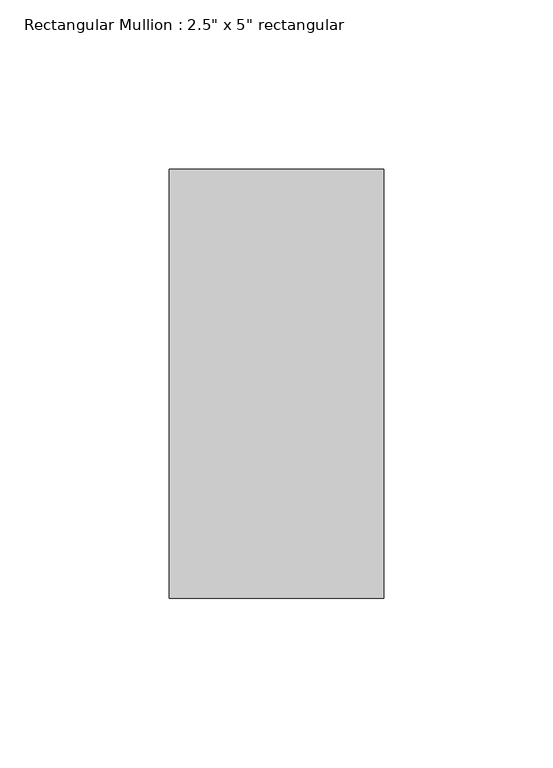
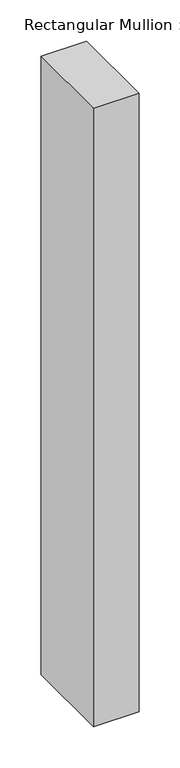
"""IFC4 building model written with IfcOpenShell, lengths in millimetres: member geometry."""

from ifc_helpers import new_model, si_unit, frame, origin, place, context, project, spatial, polyline, outline, extrude, source, transform, mapped, element, save


def member_410c6227(model_context):
    return source(origin(), model_context, "Body", "SweptSolid", [
        extrude(outline(polyline([(31.75, 63.5), (31.75, -63.5), (-31.75, -63.5), (-31.75, 63.5), (31.75, 63.5)])), frame((0.0, 0.0, -914.4), z_axis=(0.0, 0.0, 1.0), x_axis=(1.0, 0.0, 0.0)), (0.0, 0.0, 1.0), 914.4),
    ])


if __name__ == "__main__":
    model = new_model("IFC4")
    model_context = context("Model", 3, world=origin())
    ifc_project = project(units=[si_unit("LENGTHUNIT", "METRE", prefix="MILLI")], contexts=[model_context])
    site = spatial("IfcSite", under=ifc_project)
    building = spatial("IfcBuilding", under=site)
    placement = place(None, origin())
    member_shape = member_410c6227(model_context)
    element("IfcMember", 1, ObjectType="Rectangular Mullion : 2.5\" x 5\" rectangular", at=placement, inside=building, context=model_context, shape_type="MappedRepresentation", body=[
        mapped(member_shape, transform((0.0, 0.0, 0.0), x_axis=(1.0, 0.0, 0.0), y_axis=(0.0, 1.0, 0.0), z_axis=(0.0, 0.0, 1.0))),
    ])
    save(model, "model.ifc")

# Revit data of these elements
# Type "Rectangular Mullion : 2.5\" x 5\" rectangular"
#   built-in parameter 1007304 = 0.416667 (stored number, unit not read)
#   built-in parameter 1007301 = 0.104167 (stored number, unit not read)
#   built-in parameter 1007300 = 0.104167 (stored number, unit not read)
# Element 1 (IfcMember, "Rectangular Mullion : 2.5\" x 5\" rectangular")
#   Materials on its faces: "Aluminum"
# Materials
#   "Aluminum": class "Metal", colour RGB 247 247 247, transparency 0, Description = "Aluminum 6061", Cost = 0
